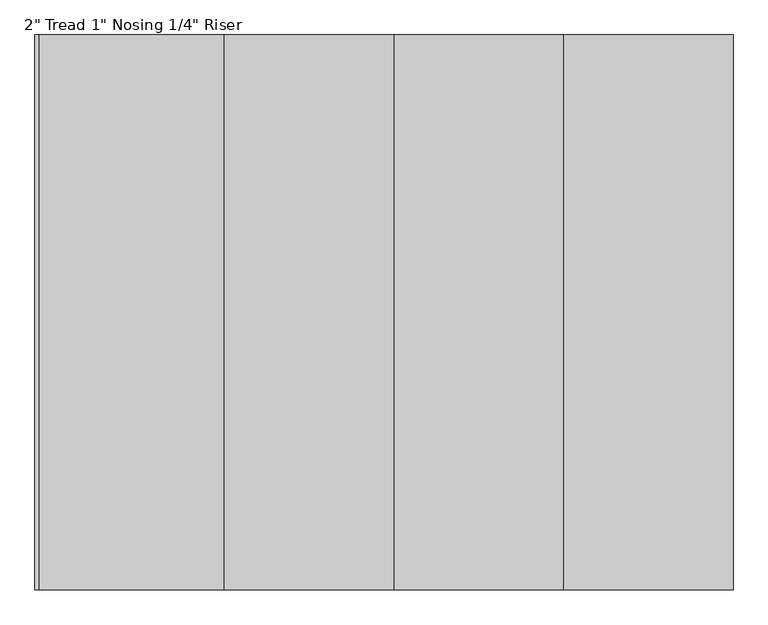
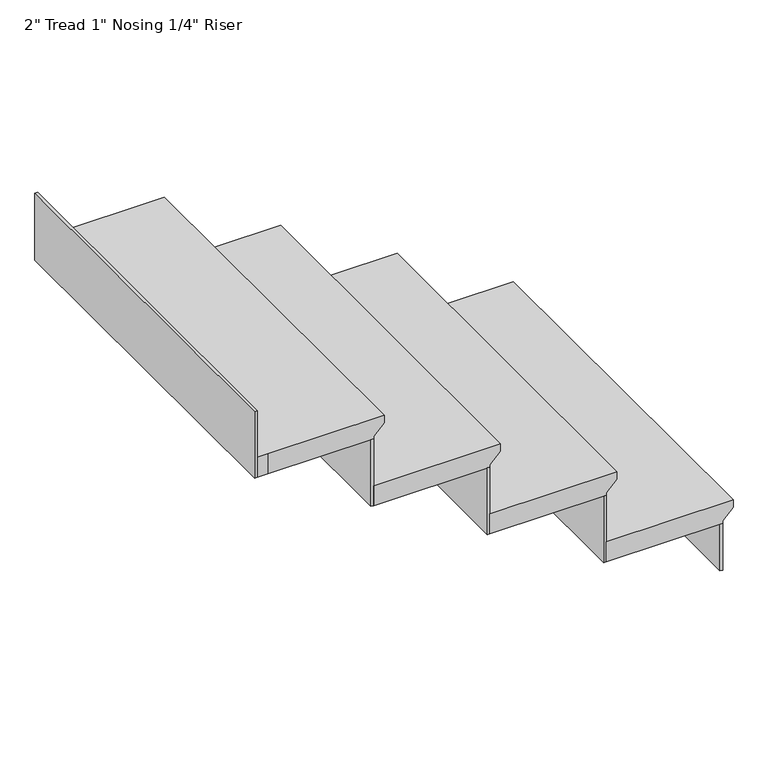
"""IFC4 building model written with IfcOpenShell, lengths in millimetres: stair flight geometry."""

from ifc_helpers import new_model, si_unit, origin, place, context, project, spatial, faceted_brep, source, transform, mapped, element, save


def stair_flight_b4bfd778(model_context):
    return source(origin(), model_context, "Body", "Brep", [
        faceted_brep([(-9079.7156858, 1045.1115003, 455.0833333), (-9079.7156858, 1045.1115003, 474.1333333), (-9079.7156858, 130.7115003, 474.1333333), (-9079.7156858, 130.7115003, 455.0833333), (-9105.1156858, 1045.1115003, 429.6833333), (-9105.1156858, 130.7115003, 429.6833333), (-9384.5156858, 1045.1115003, 474.1333333), (-9384.5156858, 130.7115003, 474.1333333), (-9105.1156858, 130.7115003, 423.3333333), (-9384.5156858, 130.7115003, 423.3333333), (-9384.5156858, 1045.1115003, 423.3333333), (-9105.1156858, 1045.1115003, 423.3333333)], [[[0, 1, 2, 3]], [[4, 0, 3, 5]], [[2, 1, 6, 7]], [[8, 9, 10, 11]], [[2, 7, 9, 8, 5, 3]], [[8, 11, 4, 5]], [[6, 1, 0, 4, 11, 10]], [[7, 6, 10, 9]]]),
        faceted_brep([(-9105.1156858, 1045.1115003, 423.3333333), (-9105.1156858, 1045.1115003, 304.8), (-9111.4656858, 1045.1115003, 304.8), (-9111.4656858, 1045.1115003, 423.3333333), (-9105.1156858, 130.7115003, 423.3333333), (-9111.4656858, 130.7115003, 423.3333333), (-9111.4656858, 130.7115003, 304.8), (-9105.1156858, 130.7115003, 304.8)], [[[0, 1, 2, 3]], [[4, 5, 6, 7]], [[1, 0, 4, 7]], [[2, 1, 7, 6]], [[3, 2, 6, 5]], [[0, 3, 5, 4]]]),
        faceted_brep([(-9384.5156858, 1045.1115003, 592.6666667), (-9384.5156858, 1045.1115003, 423.3333333), (-9390.8656858, 1045.1115003, 423.3333333), (-9390.8656858, 1045.1115003, 592.6666667), (-9384.5156858, 130.7115003, 592.6666667), (-9390.8656858, 130.7115003, 592.6666667), (-9390.8656858, 130.7115003, 423.3333333), (-9384.5156858, 130.7115003, 423.3333333)], [[[0, 1, 2, 3]], [[4, 5, 6, 7]], [[1, 0, 4, 7]], [[2, 1, 7, 6]], [[3, 2, 6, 5]], [[0, 3, 5, 4]]]),
        faceted_brep([(-9359.1156858, 130.7115003, 643.4666667), (-9359.1156858, 1045.1115003, 643.4666667), (-9663.9156858, 1045.1115003, 643.4666667), (-9663.9156858, 130.7115003, 643.4666667), (-9384.5156858, 130.7115003, 592.6666667), (-9663.9156858, 130.7115003, 592.6666667), (-9663.9156858, 1045.1115003, 592.6666667), (-9384.5156858, 1045.1115003, 592.6666667), (-9384.5156858, 130.7115003, 599.0166667), (-9359.1156858, 130.7115003, 624.4166667), (-9384.5156858, 1045.1115003, 599.0166667), (-9359.1156858, 1045.1115003, 624.4166667)], [[[0, 1, 2, 3]], [[4, 5, 6, 7]], [[0, 3, 5, 4, 8, 9]], [[4, 7, 10, 8]], [[2, 1, 11, 10, 7, 6]], [[3, 2, 6, 5]], [[11, 1, 0, 9]], [[10, 11, 9, 8]]]),
        faceted_brep([(-9663.9156858, 1045.1115003, 762.0), (-9663.9156858, 1045.1115003, 592.6666667), (-9670.2656858, 1045.1115003, 592.6666667), (-9670.2656858, 1045.1115003, 762.0), (-9663.9156858, 130.7115003, 762.0), (-9670.2656858, 130.7115003, 762.0), (-9670.2656858, 130.7115003, 592.6666667), (-9663.9156858, 130.7115003, 592.6666667)], [[[0, 1, 2, 3]], [[4, 5, 6, 7]], [[1, 0, 4, 7]], [[2, 1, 7, 6]], [[3, 2, 6, 5]], [[0, 3, 5, 4]]]),
        faceted_brep([(-9638.5156858, 130.7115003, 812.8), (-9638.5156858, 1045.1115003, 812.8), (-9943.3156858, 1045.1115003, 812.8), (-9943.3156858, 130.7115003, 812.8), (-9663.9156858, 130.7115003, 762.0), (-9943.3156858, 130.7115003, 762.0), (-9943.3156858, 1045.1115003, 762.0), (-9663.9156858, 1045.1115003, 762.0), (-9663.9156858, 130.7115003, 768.35), (-9638.5156858, 130.7115003, 793.75), (-9663.9156858, 1045.1115003, 768.35), (-9638.5156858, 1045.1115003, 793.75)], [[[0, 1, 2, 3]], [[4, 5, 6, 7]], [[0, 3, 5, 4, 8, 9]], [[4, 7, 10, 8]], [[2, 1, 11, 10, 7, 6]], [[3, 2, 6, 5]], [[11, 1, 0, 9]], [[10, 11, 9, 8]]]),
        faceted_brep([(-10222.7156858, 1045.1115003, 1100.6666667), (-10222.7156858, 1045.1115003, 931.3333333), (-10229.0656858, 1045.1115003, 931.3333333), (-10229.0656858, 1045.1115003, 1100.6666667), (-10222.7156858, 130.7115003, 1100.6666667), (-10229.0656858, 130.7115003, 1100.6666667), (-10229.0656858, 130.7115003, 931.3333333), (-10222.7156858, 130.7115003, 931.3333333)], [[[0, 1, 2, 3]], [[4, 5, 6, 7]], [[1, 0, 4, 7]], [[2, 1, 7, 6]], [[3, 2, 6, 5]], [[0, 3, 5, 4]]]),
        faceted_brep([(-9943.3156858, 1045.1115003, 931.3333333), (-9943.3156858, 1045.1115003, 762.0), (-9949.6656858, 1045.1115003, 762.0), (-9949.6656858, 1045.1115003, 931.3333333), (-9943.3156858, 130.7115003, 931.3333333), (-9949.6656858, 130.7115003, 931.3333333), (-9949.6656858, 130.7115003, 762.0), (-9943.3156858, 130.7115003, 762.0)], [[[0, 1, 2, 3]], [[4, 5, 6, 7]], [[1, 0, 4, 7]], [[2, 1, 7, 6]], [[3, 2, 6, 5]], [[0, 3, 5, 4]]]),
        faceted_brep([(-10222.7156858, 130.7115003, 982.1333333), (-10197.3156858, 130.7115003, 982.1333333), (-9917.9156858, 130.7115003, 982.1333333), (-9917.9156858, 1045.1115003, 982.1333333), (-10197.3156858, 1045.1115003, 982.1333333), (-10222.7156858, 1045.1115003, 982.1333333), (-10197.3156858, 130.7115003, 931.3333333), (-10222.7156858, 130.7115003, 931.3333333), (-10222.7156858, 1045.1115003, 931.3333333), (-10197.3156858, 1045.1115003, 931.3333333), (-9943.3156858, 1045.1115003, 931.3333333), (-9943.3156858, 130.7115003, 931.3333333), (-9943.3156858, 130.7115003, 937.6833333), (-9917.9156858, 130.7115003, 963.0833333), (-9943.3156858, 1045.1115003, 937.6833333), (-9917.9156858, 1045.1115003, 963.0833333)], [[[0, 1, 2, 3, 4, 5]], [[6, 7, 8, 9, 10, 11]], [[1, 0, 7, 6]], [[2, 1, 6, 11, 12, 13]], [[11, 10, 14, 12]], [[4, 3, 15, 14, 10, 9]], [[5, 4, 9, 8]], [[0, 5, 8, 7]], [[15, 3, 2, 13]], [[14, 15, 13, 12]]]),
    ])


if __name__ == "__main__":
    model = new_model("IFC4")
    model_context = context("Model", 3, world=origin())
    ifc_project = project(units=[si_unit("LENGTHUNIT", "METRE", prefix="MILLI")], contexts=[model_context])
    site = spatial("IfcSite", under=ifc_project)
    building = spatial("IfcBuilding", under=site)
    placement = place(None, origin())
    stair_flight_shape = stair_flight_b4bfd778(model_context)
    element("IfcStairFlight", 1, ObjectType="2\" Tread 1\" Nosing 1/4\" Riser", at=placement, inside=building, context=model_context, shape_type="MappedRepresentation", body=[
        mapped(stair_flight_shape, transform((0.0, 0.0, 0.0), x_axis=(1.0, 0.0, 0.0), y_axis=(0.0, 1.0, 0.0), z_axis=(0.0, 0.0, 1.0))),
    ])
    save(model, "model.ifc")
